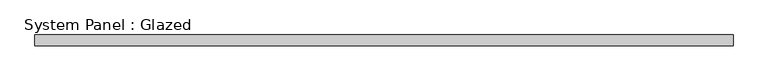
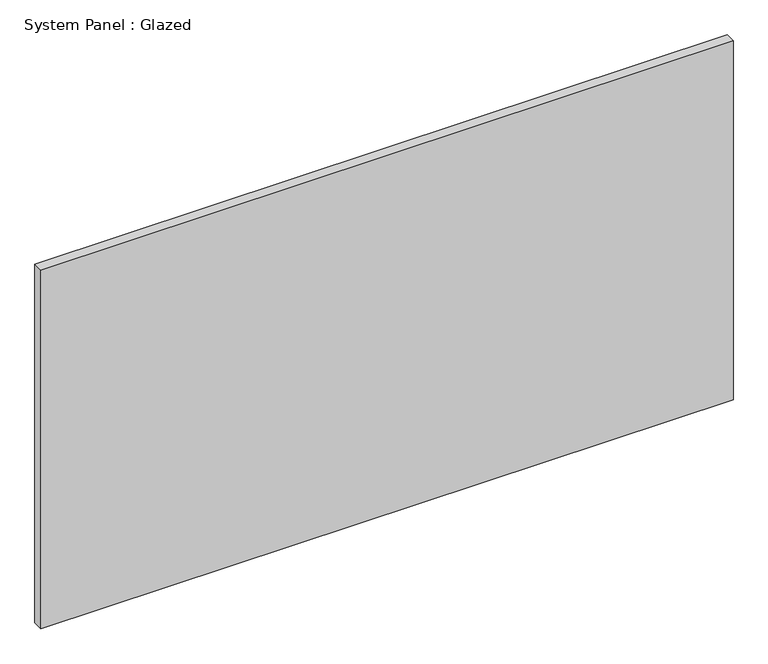
"""IFC4 building model written with IfcOpenShell, lengths in millimetres: plate geometry, System Panel : Glazed."""

from ifc_helpers import new_model, si_unit, origin, origin_with_axes, place, context, project, spatial, polyline, outline, extrude, source, transform, mapped, element, save


def system_panel_glazed_688a65a2(model_context):
    return source(origin(), model_context, "Body", "SweptSolid", [
        extrude(outline(polyline([(834.2159021, 19.05), (-834.2159021, 19.05), (-834.2159021, 44.45), (834.2159021, 44.45), (834.2159021, 19.05)])), origin_with_axes(), (0.0, 0.0, 1.0), 914.4),
    ])


if __name__ == "__main__":
    model = new_model("IFC4")
    model_context = context("Model", 3, world=origin())
    ifc_project = project(units=[si_unit("LENGTHUNIT", "METRE", prefix="MILLI")], contexts=[model_context])
    site = spatial("IfcSite", under=ifc_project)
    building = spatial("IfcBuilding", under=site)
    placement = place(None, origin())
    system_panel_glazed_shape = system_panel_glazed_688a65a2(model_context)
    element("IfcPlate", 1, ObjectType="System Panel : Glazed", at=placement, inside=building, context=model_context, shape_type="MappedRepresentation", body=[
        mapped(system_panel_glazed_shape, transform((0.0, 0.0, 0.0), x_axis=(1.0, 0.0, 0.0), y_axis=(0.0, 1.0, 0.0), z_axis=(0.0, 0.0, 1.0))),
    ])
    save(model, "model.ifc")

# Revit data of these elements
# Type "System Panel : Glazed"
#   Construction Type Id = "GSP4R"
#   Analytic Construction = "1/8 in Pilkington single glazing"
#   Visual Light Transmittance = 0.9
#   Solar Heat Gain Coefficient = 0.86
#   Heat Transfer Coefficient (U) = 6.7069 W/(m²·K)
# Element 1 (IfcPlate, "System Panel : Glazed")
#   Materials on its faces: "Glass"
# Materials
#   "Glass": class "Glass", colour RGB 0 128 192, transparency 0.75, Description = "Soda Lime Glass", Cost = 0
